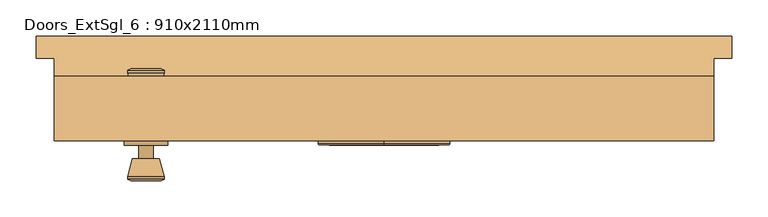
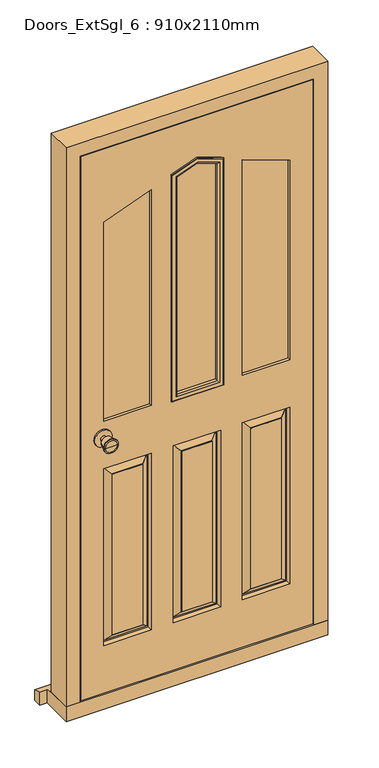
"""IFC4 building model written with IfcOpenShell, lengths in millimetres: door geometry, Doors_ExtSgl_6 : 910x2110mm."""

from ifc_helpers import new_model, si_unit, point, frame, frame_2d, origin, place, context, project, spatial, polyline, circle_curve, ellipse_curve, trimmed, segment, composite_curve, outline, extrude, faceted_brep, source, transform, mapped, element, save
from ifc_brep_helpers import plane_surface, cylinder_surface, revolved_surface, advanced_brep


def doors_extsgl_6_910x2110mm_5dc58899(model_context):
    return source(origin(), model_context, "Body", "SolidModel", [
        advanced_brep(
        [(-328.4666667, -18.4, 1000.0), (-318.4666667, -18.4, 1000.0), (-338.4666667, -18.4, 1000.0), (-307.9907991, -67.4, 1000.0), (-328.4666667, -67.4, 1000.0), (-348.9425342, -67.4, 1000.0), (-303.4666667, -65.5721319, 1000.0), (-353.4666667, -65.5721319, 1000.0), (-303.4666667, -62.1084537, 1000.0), (-353.4666667, -62.1084537, 1000.0), (-309.8304306, -37.4, 1000.0), (-347.1029027, -37.4, 1000.0), (-318.4666667, -37.4, 1000.0), (-338.4666667, -37.4, 1000.0)],
        [
            (0, 1),
            (1, 2, circle_curve(frame((-328.4666667, -18.4, 1000.0), z_axis=(0.0, 1.0, 0.0), x_axis=(-1.0, 0.0, 0.0)), 10.0)),
            (2, 0),
            (2, 1, circle_curve(frame((-328.4666667, -18.4, 1000.0), z_axis=(0.0, 1.0, 0.0), x_axis=(-1.0, 0.0, 0.0)), 10.0)),
            (3, 4),
            (4, 5),
            (5, 3, circle_curve(frame((-328.4666667, -67.4, 1000.0), z_axis=(0.0, -1.0, 0.0), x_axis=(-1.0, 0.0, 0.0)), 20.4758676)),
            (3, 5, circle_curve(frame((-328.4666667, -67.4, 1000.0), z_axis=(0.0, -1.0, 0.0), x_axis=(-1.0, 0.0, 0.0)), 20.4758676)),
            (6, 3),
            (5, 7),
            (7, 6, circle_curve(frame((-328.4666667, -65.5721319, 1000.0), z_axis=(0.0, -1.0, 0.0), x_axis=(-1.0, 0.0, 0.0)), 25.0)),
            (6, 7, circle_curve(frame((-328.4666667, -65.5721319, 1000.0), z_axis=(0.0, -1.0, 0.0), x_axis=(-1.0, 0.0, 0.0)), 25.0)),
            (8, 6),
            (7, 9),
            (9, 8, circle_curve(frame((-328.4666667, -62.1084537, 1000.0), z_axis=(0.0, -1.0, 0.0), x_axis=(-1.0, 0.0, 0.0)), 25.0)),
            (8, 9, circle_curve(frame((-328.4666667, -62.1084537, 1000.0), z_axis=(0.0, -1.0, 0.0), x_axis=(-1.0, 0.0, 0.0)), 25.0)),
            (10, 8),
            (9, 11),
            (11, 10, circle_curve(frame((-328.4666667, -37.4, 1000.0), z_axis=(0.0, -1.0, 0.0), x_axis=(-1.0, 0.0, 0.0)), 18.636236)),
            (10, 11, circle_curve(frame((-328.4666667, -37.4, 1000.0), z_axis=(0.0, -1.0, 0.0), x_axis=(-1.0, 0.0, 0.0)), 18.636236)),
            (12, 10),
            (11, 13),
            (13, 12, circle_curve(frame((-328.4666667, -37.4, 1000.0), z_axis=(0.0, -1.0, 0.0), x_axis=(-1.0, 0.0, 0.0)), 10.0)),
            (12, 13, circle_curve(frame((-328.4666667, -37.4, 1000.0), z_axis=(0.0, -1.0, 0.0), x_axis=(-1.0, 0.0, 0.0)), 10.0)),
            (1, 12),
            (13, 2),
        ],
        [
            plane_surface(frame((-328.4666667, -18.4, 1000.0), z_axis=(0.0, 1.0, 0.0), x_axis=(-1.0, 0.0, 0.0))),
            plane_surface(frame((-328.4666667, -67.4, 1000.0), z_axis=(0.0, -1.0, 0.0), x_axis=(-1.0, 0.0, 0.0))),
            revolved_surface(polyline([(-348.9425342, -67.4, 1000.0), (-353.4666667, -65.5721319, 1000.0)]), (-328.4666667, -18.4, 1000.0), (0.0, 1.0, 0.0)),
            cylinder_surface(frame((-328.4666667, -18.4, 1000.0), z_axis=(0.0, 1.0, 0.0), x_axis=(-1.0, 0.0, 0.0)), 25.0),
            revolved_surface(polyline([(-353.4666667, -62.1084537, 1000.0), (-347.1029027, -37.4, 1000.0)]), (-328.4666667, -18.4, 1000.0), (0.0, 1.0, 0.0)),
            plane_surface(frame((-328.4666667, -37.4, 1000.0), z_axis=(0.0, 1.0, 0.0), x_axis=(-1.0, 0.0, 0.0))),
            cylinder_surface(frame((-328.4666667, -18.4, 1000.0), z_axis=(0.0, 1.0, 0.0), x_axis=(-1.0, 0.0, 0.0)), 10.0),
        ],
        [
            (0, [[1, 2, 3]]),
            (0, [[-3, 4, -1]]),
            (1, [[5, 6, 7]]),
            (1, [[-6, -5, 8]]),
            (2, [[9, -7, 10, 11]]),
            (2, [[-10, -8, -9, 12]]),
            (3, [[13, -11, 14, 15]]),
            (3, [[-14, -12, -13, 16]]),
            (4, [[17, -15, 18, 19]]),
            (4, [[-18, -16, -17, 20]]),
            (5, [[21, -19, 22, 23]]),
            (5, [[-22, -20, -21, 24]]),
            (6, [[25, -23, 26, -2]]),
            (6, [[-26, -24, -25, -4]]),
        ],
    ),
        extrude(outline(composite_curve([segment(trimmed(circle_curve(frame_2d((1000.0, -328.4666667)), 30.0), [point((1000.0, -358.4666667))], [point((1000.0, -298.4666667))], False, "CARTESIAN"), True, "CONTINUOUS"), segment(trimmed(circle_curve(frame_2d((1000.0, -328.4666667)), 30.0), [point((1000.0, -298.4666667))], [point((1000.0, -358.4666667))], False, "CARTESIAN"), True, "CONTINUOUS")], self_intersect=False)), frame((0.0, -18.4, 0.0), z_axis=(0.0, 1.0, 0.0), x_axis=(0.0, 0.0, 1.0)), (0.0, 0.0, 1.0), 6.0),
        advanced_brep(
        [(-328.4666667, 37.6, 1000.0), (-338.4666667, 37.6, 1000.0), (-318.4666667, 37.6, 1000.0), (-307.9907991, 86.6, 1000.0), (-348.9425342, 86.6, 1000.0), (-328.4666667, 86.6, 1000.0), (-303.4666667, 84.7721319, 1000.0), (-353.4666667, 84.7721319, 1000.0), (-303.4666667, 81.3084537, 1000.0), (-353.4666667, 81.3084537, 1000.0), (-309.8304306, 56.6, 1000.0), (-347.1029027, 56.6, 1000.0), (-318.4666667, 56.6, 1000.0), (-338.4666667, 56.6, 1000.0)],
        [
            (0, 1),
            (1, 2, circle_curve(frame((-328.4666667, 37.6, 1000.0), z_axis=(0.0, -1.0, 0.0), x_axis=(-1.0, 0.0, 0.0)), 10.0)),
            (2, 0),
            (2, 1, circle_curve(frame((-328.4666667, 37.6, 1000.0), z_axis=(0.0, -1.0, 0.0), x_axis=(-1.0, 0.0, 0.0)), 10.0)),
            (3, 4, circle_curve(frame((-328.4666667, 86.6, 1000.0), z_axis=(0.0, 1.0, 0.0), x_axis=(-1.0, 0.0, 0.0)), 20.4758676)),
            (4, 5),
            (5, 3),
            (4, 3, circle_curve(frame((-328.4666667, 86.6, 1000.0), z_axis=(0.0, 1.0, 0.0), x_axis=(-1.0, 0.0, 0.0)), 20.4758676)),
            (6, 7, circle_curve(frame((-328.4666667, 84.7721319, 1000.0), z_axis=(0.0, 1.0, 0.0), x_axis=(-1.0, 0.0, 0.0)), 25.0)),
            (7, 4),
            (3, 6),
            (7, 6, circle_curve(frame((-328.4666667, 84.7721319, 1000.0), z_axis=(0.0, 1.0, 0.0), x_axis=(-1.0, 0.0, 0.0)), 25.0)),
            (8, 9, circle_curve(frame((-328.4666667, 81.3084537, 1000.0), z_axis=(0.0, 1.0, 0.0), x_axis=(-1.0, 0.0, 0.0)), 25.0)),
            (9, 7),
            (6, 8),
            (9, 8, circle_curve(frame((-328.4666667, 81.3084537, 1000.0), z_axis=(0.0, 1.0, 0.0), x_axis=(-1.0, 0.0, 0.0)), 25.0)),
            (10, 11, circle_curve(frame((-328.4666667, 56.6, 1000.0), z_axis=(0.0, 1.0, 0.0), x_axis=(-1.0, 0.0, 0.0)), 18.636236)),
            (11, 9),
            (8, 10),
            (11, 10, circle_curve(frame((-328.4666667, 56.6, 1000.0), z_axis=(0.0, 1.0, 0.0), x_axis=(-1.0, 0.0, 0.0)), 18.636236)),
            (12, 13, circle_curve(frame((-328.4666667, 56.6, 1000.0), z_axis=(0.0, 1.0, 0.0), x_axis=(-1.0, 0.0, 0.0)), 10.0)),
            (13, 11),
            (10, 12),
            (13, 12, circle_curve(frame((-328.4666667, 56.6, 1000.0), z_axis=(0.0, 1.0, 0.0), x_axis=(-1.0, 0.0, 0.0)), 10.0)),
            (1, 13),
            (12, 2),
        ],
        [
            plane_surface(frame((-328.4666667, 37.6, 1000.0), z_axis=(0.0, -1.0, 0.0), x_axis=(-1.0, 0.0, 0.0))),
            plane_surface(frame((-328.4666667, 86.6, 1000.0), z_axis=(0.0, 1.0, 0.0), x_axis=(-1.0, 0.0, 0.0))),
            revolved_surface(polyline([(-348.9425342, 86.6, 1000.0), (-353.4666667, 84.7721319, 1000.0)]), (-328.4666667, 37.6, 1000.0), (0.0, -1.0, 0.0)),
            cylinder_surface(frame((-328.4666667, 37.6, 1000.0), z_axis=(0.0, -1.0, 0.0), x_axis=(-1.0, 0.0, 0.0)), 25.0),
            revolved_surface(polyline([(-353.4666667, 81.3084537, 1000.0), (-347.1029027, 56.6, 1000.0)]), (-328.4666667, 37.6, 1000.0), (0.0, -1.0, 0.0)),
            plane_surface(frame((-328.4666667, 56.6, 1000.0), z_axis=(0.0, -1.0, 0.0), x_axis=(-1.0, 0.0, 0.0))),
            cylinder_surface(frame((-328.4666667, 37.6, 1000.0), z_axis=(0.0, -1.0, 0.0), x_axis=(-1.0, 0.0, 0.0)), 10.0),
        ],
        [
            (0, [[1, 2, 3]]),
            (0, [[-3, 4, -1]]),
            (1, [[5, 6, 7]]),
            (1, [[8, -7, -6]]),
            (2, [[9, 10, -5, 11]]),
            (2, [[12, -11, -8, -10]]),
            (3, [[13, 14, -9, 15]]),
            (3, [[16, -15, -12, -14]]),
            (4, [[17, 18, -13, 19]]),
            (4, [[20, -19, -16, -18]]),
            (5, [[21, 22, -17, 23]]),
            (5, [[24, -23, -20, -22]]),
            (6, [[-2, 25, -21, 26]]),
            (6, [[-4, -26, -24, -25]]),
        ],
    ),
        extrude(outline(composite_curve([segment(trimmed(circle_curve(frame_2d((1000.0, -328.4666667)), 30.0), [point((1000.0, -358.4666667))], [point((1000.0, -298.4666667))], False, "CARTESIAN"), True, "CONTINUOUS"), segment(trimmed(circle_curve(frame_2d((1000.0, -328.4666667)), 30.0), [point((1000.0, -298.4666667))], [point((1000.0, -358.4666667))], False, "CARTESIAN"), True, "CONTINUOUS")], self_intersect=False)), frame((0.0, 31.6, 0.0), z_axis=(0.0, 1.0, 0.0), x_axis=(0.0, 0.0, 1.0)), (0.0, 0.0, 1.0), 6.0),
        faceted_brep([(384.5333333, 76.6, 54.5), (455.0333333, 76.6, 54.5), (455.0333333, -12.4, 54.5), (406.5333333, -12.4, 54.5), (406.5333333, 34.6, 54.5), (384.5333333, 34.6, 54.5), (384.5333333, 76.6, 2039.5), (-384.4666667, 76.6, 2039.5), (-384.4666667, 76.6, 54.5), (-454.9666667, 76.6, 54.5), (-454.9666667, 76.6, 2110.0), (455.0333333, 76.6, 2110.0), (455.0333333, -12.4, 2110.0), (-454.9666667, -12.4, 2110.0), (-454.9666667, -12.4, 54.5), (-406.4666667, -12.4, 54.5), (-406.4666667, -12.4, 2061.5), (406.5333333, -12.4, 2061.5), (406.5333333, 34.6, 2061.5), (-406.4666667, 34.6, 2061.5), (-406.4666667, 34.6, 54.5), (-384.4666667, 34.6, 54.5), (-384.4666667, 34.6, 2039.5), (384.5333333, 34.6, 2039.5)], [[[0, 1, 2, 3, 4, 5]], [[1, 0, 6, 7, 8, 9, 10, 11]], [[2, 1, 11, 12]], [[3, 2, 12, 13, 14, 15, 16, 17]], [[4, 3, 17, 18]], [[5, 4, 18, 19, 20, 21, 22, 23]], [[0, 5, 23, 6]], [[8, 7, 22, 21]], [[9, 8, 21, 20, 15, 14]], [[10, 9, 14, 13]], [[16, 15, 20, 19]], [[11, 10, 13, 12]], [[17, 16, 19, 18]], [[7, 6, 23, 22]]]),
        faceted_brep([(403.5333333, -12.4, 58.5), (403.5333333, -12.4, 2058.5), (-404.3916961, -12.4, 2058.5), (-404.3916961, -12.4, 58.5), (-82.8, -12.4, 1058.5), (-82.8, -12.4, 1878.3511323), (0.0333333, -12.4, 1908.5), (82.8666667, -12.4, 1878.3511323), (82.8666667, -12.4, 1058.5), (323.5333333, -12.4, 1058.5), (157.8666667, -12.4, 1058.5), (157.8666667, -12.4, 1851.0533647), (323.5333333, -12.4, 1790.7556292), (-157.8, -12.4, 1851.0533647), (-157.8, -12.4, 1058.5), (-323.4666667, -12.4, 1058.5), (-323.4666667, -12.4, 1790.7556292), (-157.8, -12.4, 883.5), (-157.8, -12.4, 233.5), (-323.4666667, -12.4, 233.5), (-323.4666667, -12.4, 883.5), (323.5333333, -12.4, 883.5), (323.5333333, -12.4, 233.5), (157.8666667, -12.4, 233.5), (157.8666667, -12.4, 883.5), (82.8666667, -12.4, 883.5), (82.8666667, -12.4, 233.5), (-82.8, -12.4, 233.5), (-82.8, -12.4, 883.5), (-187.8, -12.4, 263.5), (-187.8, -12.4, 853.5), (-293.4666667, -12.4, 853.5), (-293.4666667, -12.4, 263.5), (293.5333333, -12.4, 263.5), (293.5333333, -12.4, 853.5), (187.8666667, -12.4, 853.5), (187.8666667, -12.4, 263.5), (52.8666667, -12.4, 263.5), (52.8666667, -12.4, 853.5), (-52.8, -12.4, 853.5), (-52.8, -12.4, 263.5), (403.5333333, 31.6, 58.5), (-404.3916961, 31.6, 58.5), (-404.3916961, 31.6, 2058.5), (403.5333333, 31.6, 2058.5), (-82.8, 31.6, 1058.5), (82.8666667, 31.6, 1058.5), (82.8666667, 31.6, 1878.3511323), (0.0333333, 31.6, 1908.5), (-82.8, 31.6, 1878.3511323), (323.5333333, 31.6, 1058.5), (323.5333333, 31.6, 1790.7556292), (157.8666667, 31.6, 1851.0533647), (157.8666667, 31.6, 1058.5), (-157.8, 31.6, 1851.0533647), (-323.4666667, 31.6, 1790.7556292), (-323.4666667, 31.6, 1058.5), (-157.8, 31.6, 1058.5), (157.8666667, 31.6, 883.5), (157.8666667, 31.6, 233.5), (323.5333333, 31.6, 233.5), (323.5333333, 31.6, 883.5), (-323.4666667, 31.6, 883.5), (-323.4666667, 31.6, 233.5), (-157.8, 31.6, 233.5), (-157.8, 31.6, 883.5), (-82.8, 31.6, 883.5), (-82.8, 31.6, 233.5), (82.8666667, 31.6, 233.5), (82.8666667, 31.6, 883.5), (187.8666667, 31.6, 263.5), (187.8666667, 31.6, 853.5), (293.5333333, 31.6, 853.5), (293.5333333, 31.6, 263.5), (-293.4666667, 31.6, 263.5), (-293.4666667, 31.6, 853.5), (-187.8, 31.6, 853.5), (-187.8, 31.6, 263.5), (-52.8, 31.6, 263.5), (-52.8, 31.6, 853.5), (52.8666667, 31.6, 853.5), (52.8666667, 31.6, 263.5), (160.8666667, 16.6, 880.5), (160.8666667, 16.6, 236.5), (185.8666667, 30.6, 855.5), (185.8666667, 30.6, 261.5), (165.8666667, 16.6, 241.5), (165.8666667, 16.6, 875.5), (187.8666667, 30.6, 263.5), (187.8666667, 30.6, 853.5), (320.5333333, 16.6, 236.5), (295.5333333, 30.6, 261.5), (315.5333333, 16.6, 241.5), (293.5333333, 30.6, 263.5), (320.5333333, 16.6, 880.5), (295.5333333, 30.6, 855.5), (315.5333333, 16.6, 875.5), (293.5333333, 30.6, 853.5), (-320.4666667, 16.6, 880.5), (-320.4666667, 16.6, 236.5), (-295.4666667, 30.6, 855.5), (-295.4666667, 30.6, 261.5), (-315.4666667, 16.6, 241.5), (-315.4666667, 16.6, 875.5), (-293.4666667, 30.6, 263.5), (-293.4666667, 30.6, 853.5), (-160.8, 16.6, 236.5), (-185.8, 30.6, 261.5), (-165.8, 16.6, 241.5), (-187.8, 30.6, 263.5), (-160.8, 16.6, 880.5), (-185.8, 30.6, 855.5), (-165.8, 16.6, 875.5), (-187.8, 30.6, 853.5), (-187.8, -11.4, 263.5), (-187.8, -11.4, 853.5), (-165.8, 2.6, 241.5), (-165.8, 2.6, 875.5), (-185.8, -11.4, 855.5), (-185.8, -11.4, 261.5), (-160.8, 2.6, 880.5), (-160.8, 2.6, 236.5), (-293.4666667, -11.4, 853.5), (-315.4666667, 2.6, 875.5), (-295.4666667, -11.4, 855.5), (-320.4666667, 2.6, 880.5), (-293.4666667, -11.4, 263.5), (-315.4666667, 2.6, 241.5), (-295.4666667, -11.4, 261.5), (-320.4666667, 2.6, 236.5), (320.5333333, 2.6, 880.5), (320.5333333, 2.6, 236.5), (295.5333333, -11.4, 855.5), (295.5333333, -11.4, 261.5), (315.5333333, 2.6, 241.5), (315.5333333, 2.6, 875.5), (293.5333333, -11.4, 263.5), (293.5333333, -11.4, 853.5), (160.8666667, 2.6, 236.5), (185.8666667, -11.4, 261.5), (165.8666667, 2.6, 241.5), (187.8666667, -11.4, 263.5), (160.8666667, 2.6, 880.5), (185.8666667, -11.4, 855.5), (165.8666667, 2.6, 875.5), (187.8666667, -11.4, 853.5), (-52.8, 30.6, 263.5), (-52.8, 30.6, 853.5), (-74.8, 16.6, 241.5), (-74.8, 16.6, 875.5), (-54.8, 30.6, 855.5), (-54.8, 30.6, 261.5), (-79.8, 16.6, 880.5), (-79.8, 16.6, 236.5), (52.8666667, 30.6, 853.5), (74.8666667, 16.6, 875.5), (54.8666667, 30.6, 855.5), (79.8666667, 16.6, 880.5), (52.8666667, 30.6, 263.5), (74.8666667, 16.6, 241.5), (54.8666667, 30.6, 261.5), (79.8666667, 16.6, 236.5), (79.8666667, 2.6, 880.5), (79.8666667, 2.6, 236.5), (54.8666667, -11.4, 855.5), (54.8666667, -11.4, 261.5), (74.8666667, 2.6, 241.5), (74.8666667, 2.6, 875.5), (52.8666667, -11.4, 263.5), (52.8666667, -11.4, 853.5), (-79.8, 2.6, 236.5), (-54.8, -11.4, 261.5), (-74.8, 2.6, 241.5), (-52.8, -11.4, 263.5), (-79.8, 2.6, 880.5), (-54.8, -11.4, 855.5), (-74.8, 2.6, 875.5), (-52.8, -11.4, 853.5)], [[[0, 1, 2, 3], [4, 5, 6, 7, 8], [9, 10, 11, 12], [13, 14, 15, 16], [17, 18, 19, 20], [21, 22, 23, 24], [25, 26, 27, 28]], [[29, 30, 31, 32]], [[33, 34, 35, 36]], [[37, 38, 39, 40]], [[41, 42, 43, 44], [45, 46, 47, 48, 49], [50, 51, 52, 53], [54, 55, 56, 57], [58, 59, 60, 61], [62, 63, 64, 65], [66, 67, 68, 69]], [[70, 71, 72, 73]], [[74, 75, 76, 77]], [[78, 79, 80, 81]], [[1, 0, 41, 44]], [[2, 1, 44, 43]], [[3, 2, 43, 42]], [[0, 3, 42, 41]], [[5, 4, 45, 49]], [[6, 5, 49, 48]], [[7, 6, 48, 47]], [[8, 7, 47, 46]], [[4, 8, 46, 45]], [[10, 9, 50, 53]], [[11, 10, 53, 52]], [[12, 11, 52, 51]], [[9, 12, 51, 50]], [[14, 13, 54, 57]], [[15, 14, 57, 56]], [[16, 15, 56, 55]], [[13, 16, 55, 54]], [[82, 83, 59, 58]], [[84, 85, 86, 87]], [[70, 88, 89, 71]], [[59, 83, 90, 60]], [[86, 85, 91, 92]], [[88, 70, 73, 93]], [[60, 90, 94, 61]], [[92, 91, 95, 96]], [[93, 73, 72, 97]], [[82, 58, 61, 94]], [[83, 82, 94, 90], [87, 86, 92, 96]], [[84, 87, 96, 95]], [[85, 84, 95, 91], [89, 88, 93, 97]], [[71, 89, 97, 72]], [[98, 99, 63, 62]], [[100, 101, 102, 103]], [[74, 104, 105, 75]], [[63, 99, 106, 64]], [[102, 101, 107, 108]], [[104, 74, 77, 109]], [[64, 106, 110, 65]], [[108, 107, 111, 112]], [[109, 77, 76, 113]], [[98, 62, 65, 110]], [[99, 98, 110, 106], [103, 102, 108, 112]], [[100, 103, 112, 111]], [[101, 100, 111, 107], [105, 104, 109, 113]], [[75, 105, 113, 76]], [[114, 115, 30, 29]], [[116, 117, 118, 119]], [[17, 120, 121, 18]], [[30, 115, 122, 31]], [[118, 117, 123, 124]], [[120, 17, 20, 125]], [[31, 122, 126, 32]], [[124, 123, 127, 128]], [[125, 20, 19, 129]], [[114, 29, 32, 126]], [[119, 118, 124, 128], [115, 114, 126, 122]], [[116, 119, 128, 127]], [[121, 120, 125, 129], [117, 116, 127, 123]], [[18, 121, 129, 19]], [[130, 131, 22, 21]], [[132, 133, 134, 135]], [[33, 136, 137, 34]], [[22, 131, 138, 23]], [[134, 133, 139, 140]], [[136, 33, 36, 141]], [[23, 138, 142, 24]], [[140, 139, 143, 144]], [[141, 36, 35, 145]], [[130, 21, 24, 142]], [[131, 130, 142, 138], [135, 134, 140, 144]], [[132, 135, 144, 143]], [[133, 132, 143, 139], [137, 136, 141, 145]], [[34, 137, 145, 35]], [[146, 147, 79, 78]], [[148, 149, 150, 151]], [[66, 152, 153, 67]], [[79, 147, 154, 80]], [[150, 149, 155, 156]], [[152, 66, 69, 157]], [[80, 154, 158, 81]], [[156, 155, 159, 160]], [[157, 69, 68, 161]], [[146, 78, 81, 158]], [[151, 150, 156, 160], [147, 146, 158, 154]], [[148, 151, 160, 159]], [[153, 152, 157, 161], [149, 148, 159, 155]], [[67, 153, 161, 68]], [[162, 163, 26, 25]], [[164, 165, 166, 167]], [[37, 168, 169, 38]], [[26, 163, 170, 27]], [[166, 165, 171, 172]], [[168, 37, 40, 173]], [[27, 170, 174, 28]], [[172, 171, 175, 176]], [[173, 40, 39, 177]], [[162, 25, 28, 174]], [[163, 162, 174, 170], [167, 166, 172, 176]], [[164, 167, 176, 175]], [[165, 164, 175, 171], [169, 168, 173, 177]], [[38, 169, 177, 39]]]),
        faceted_brep([(480.0333333, 131.6, 0.0), (480.0333333, 131.6, 38.5947221), (480.0333333, 101.6, 47.2703282), (480.0333333, 101.6, 0.0), (-479.9666667, 131.6, 38.5947221), (-479.9666667, 131.6, 0.0), (-479.9666667, 101.6, 0.0), (-479.9666667, 101.6, 47.2703282), (455.0333333, 101.6, 0.0), (455.0333333, -12.4, 0.0), (-454.9666667, -12.4, 0.0), (-454.9666667, 101.6, 0.0), (-454.9666667, 101.6, 47.2703282), (-454.9666667, 76.6, 54.5), (455.0333333, 76.6, 54.5), (455.0333333, 101.6, 47.2703282), (-454.9666667, -12.4, 54.5), (455.0333333, -12.4, 54.5)], [[[0, 1, 2, 3]], [[4, 5, 6, 7]], [[5, 0, 3, 8, 9, 10, 11, 6]], [[1, 0, 5, 4]], [[1, 4, 7, 12, 13, 14, 15, 2]], [[13, 16, 17, 14]], [[16, 10, 9, 17]], [[12, 11, 10, 16, 13]], [[11, 12, 7, 6]], [[8, 15, 14, 17, 9]], [[15, 8, 3, 2]]]),
        extrude(outline(polyline([(1058.5, -82.8), (1058.5, 82.8666667), (1878.3511323, 82.8666667), (1908.5, 0.0333333), (1878.3511323, -82.8), (1058.5, -82.8)])), frame((0.0, -2.4, 0.0), z_axis=(0.0, 1.0, 0.0), x_axis=(0.0, 0.0, 1.0)), (0.0, 0.0, 1.0), 24.0),
        extrude(outline(polyline([(1790.7556292, 323.5333333), (1851.0533647, 157.8666667), (1058.5, 157.8666667), (1058.5, 323.5333333), (1790.7556292, 323.5333333)])), frame((0.0, -2.4, 0.0), z_axis=(0.0, 1.0, 0.0), x_axis=(0.0, 0.0, 1.0)), (0.0, 0.0, 1.0), 24.0),
        extrude(outline(polyline([(1058.5, -157.8), (1851.0533647, -157.8), (1790.7556292, -323.4666667), (1058.5, -323.4666667), (1058.5, -157.8)])), frame((0.0, -2.4, 0.0), z_axis=(0.0, 1.0, 0.0), x_axis=(0.0, 0.0, 1.0)), (0.0, 0.0, 1.0), 24.0),
        advanced_brep(
        [(-90.8, 35.6, 1050.5), (-90.8, 31.6, 1050.5), (-90.8, 31.6, 1883.9527926), (-90.8, 35.6, 1883.9527926), (-88.8, 37.6, 1052.5), (-88.8, 37.6, 1882.5523775), (-70.8, 32.6, 1070.5), (-75.8, 37.6, 1065.5), (-75.8, 37.6, 1873.4496795), (-70.8, 32.6, 1869.9486418), (-70.8, 21.6, 1070.5), (-70.8, 21.6, 1869.9486418), (-82.8, 31.6, 1058.5), (-82.8, 21.6, 1058.5), (-82.8, 21.6, 1878.3511323), (-82.8, 31.6, 1878.3511323), (0.0333333, 31.6, 1917.0134222), (0.0333333, 35.6, 1917.0134222), (0.0333333, 37.6, 1914.8850666), (0.0333333, 37.6, 1901.0507556), (0.0333333, 32.6, 1895.7298667), (0.0333333, 21.6, 1895.7298667), (0.0333333, 21.6, 1908.5), (0.0333333, 31.6, 1908.5), (90.8666667, 31.6, 1883.9527926), (90.8666667, 35.6, 1883.9527926), (88.8666667, 37.6, 1882.5523775), (88.8666667, 37.6, 1052.5), (75.8666667, 37.6, 1873.4496795), (75.8666667, 37.6, 1065.5), (70.8666667, 32.6, 1869.9486418), (70.8666667, 21.6, 1869.9486418), (82.8666667, 21.6, 1878.3511323), (82.8666667, 21.6, 1058.5), (70.8666667, 21.6, 1070.5), (82.8666667, 31.6, 1878.3511323), (90.8666667, 31.6, 1050.5), (82.8666667, 31.6, 1058.5), (90.8666667, 35.6, 1050.5), (70.8666667, 32.6, 1070.5)],
        [
            (0, 1),
            (1, 2),
            (2, 3),
            (3, 0),
            (4, 0, ellipse_curve(frame((-88.8, 35.6, 1052.5), z_axis=(-0.7071067811865476, 0.0, 0.7071067811865474), x_axis=(-0.7071067811865472, 0.0, -0.7071067811865478)), 2.8284271, 2.0)),
            (3, 5, ellipse_curve(frame((-88.8, 35.6, 1882.5523775), z_axis=(-0.5735764363510456, 0.0, -0.8191520442889918), x_axis=(0.8191520442889916, 0.0, -0.5735764363510464)), 2.4415492, 2.0)),
            (5, 4),
            (6, 7, ellipse_curve(frame((-75.8, 32.6, 1065.5), z_axis=(-0.7071067811865476, 0.0, 0.7071067811865474), x_axis=(-0.7071067811865472, 0.0, -0.7071067811865478)), 7.0710678, 5.0)),
            (7, 8),
            (8, 9, ellipse_curve(frame((-75.8, 32.6, 1873.4496795), z_axis=(-0.5735764363510456, 0.0, -0.8191520442889918), x_axis=(0.8191520442889916, 0.0, -0.5735764363510464)), 6.1038729, 5.0)),
            (9, 6),
            (10, 6),
            (9, 11),
            (11, 10),
            (12, 13),
            (13, 14),
            (14, 15),
            (15, 12),
            (2, 16),
            (16, 17),
            (17, 3),
            (17, 18, ellipse_curve(frame((0.0333333, 35.6, 1914.8850666), z_axis=(-1.0, 0.0, 0.0), x_axis=(0.0, 0.0, -1.0)), 2.1283555, 2.0)),
            (18, 5),
            (8, 19),
            (19, 20, ellipse_curve(frame((0.0333333, 32.6, 1901.0507556), z_axis=(-1.0, 0.0, 0.0), x_axis=(0.0, 0.0, -1.0)), 5.3208889, 5.0)),
            (20, 9),
            (20, 21),
            (21, 11),
            (14, 22),
            (22, 23),
            (23, 15),
            (16, 24),
            (24, 25),
            (25, 17),
            (25, 26, ellipse_curve(frame((88.8666667, 35.6, 1882.5523775), z_axis=(-0.573576436351046, 0.0, 0.8191520442889917), x_axis=(-0.8191520442889921, 0.0, -0.5735764363510458)), 2.4415492, 2.0)),
            (26, 18),
            (26, 27),
            (27, 4),
            (28, 19),
            (7, 29),
            (29, 28),
            (28, 30, ellipse_curve(frame((75.8666667, 32.6, 1873.4496795), z_axis=(-0.573576436351046, 0.0, 0.8191520442889917), x_axis=(-0.8191520442889921, 0.0, -0.5735764363510458)), 6.1038729, 5.0)),
            (30, 20),
            (30, 31),
            (31, 21),
            (32, 22),
            (13, 33),
            (33, 32),
            (31, 34),
            (34, 10),
            (32, 35),
            (35, 23),
            (1, 36),
            (36, 24),
            (35, 37),
            (37, 12),
            (36, 38),
            (38, 25),
            (38, 27, ellipse_curve(frame((88.8666667, 35.6, 1052.5), z_axis=(0.7071067811865475, 0.0, 0.7071067811865476), x_axis=(-0.7071067811865475, 0.0, 0.7071067811865475)), 2.8284271, 2.0)),
            (29, 39, ellipse_curve(frame((75.8666667, 32.6, 1065.5), z_axis=(0.7071067811865475, 0.0, 0.7071067811865476), x_axis=(-0.7071067811865475, 0.0, 0.7071067811865475)), 7.0710678, 5.0)),
            (39, 30),
            (39, 34),
            (33, 37),
            (0, 38),
            (6, 39),
        ],
        [
            plane_surface(frame((-90.8, 31.6, 1050.5), z_axis=(-1.0, 0.0, 0.0), x_axis=(0.0, 0.0, 1.0))),
            cylinder_surface(frame((-88.8, 35.6, 1058.5), z_axis=(0.0, 0.0, -1.0), x_axis=(-1.0, 0.0, 0.0)), 2.0),
            cylinder_surface(frame((-75.8, 32.6, 1058.5), z_axis=(0.0, 0.0, -1.0), x_axis=(-1.0, 0.0, 0.0)), 5.0),
            plane_surface(frame((-70.8, 32.6, 1070.5), z_axis=(1.0, 0.0, 0.0), x_axis=(0.0, 0.0, 1.0))),
            plane_surface(frame((-82.8, 21.6, 1058.5), z_axis=(-1.0, 0.0, 0.0), x_axis=(0.0, 0.0, 1.0))),
            plane_surface(frame((-90.8, 31.6, 1883.9527926), z_axis=(-0.34202014332566827, 0.0, 0.9396926207859086), x_axis=(0.9396926207859086, 0.0, 0.34202014332566827))),
            cylinder_surface(frame((-84.8521209, 35.6, 1883.989288), z_axis=(-0.9396926207859082, 0.0, -0.34202014332566943), x_axis=(-0.34202014332566943, 0.0, 0.9396926207859082)), 2.0),
            cylinder_surface(frame((-80.405859, 32.6, 1871.7732839), z_axis=(-0.9396926207859082, 0.0, -0.34202014332566943), x_axis=(-0.34202014332566943, 0.0, 0.9396926207859082)), 5.0),
            plane_surface(frame((-70.8, 32.6, 1869.9486418), z_axis=(0.34202014332567066, 0.0, -0.9396926207859078), x_axis=(0.9396926207859078, 0.0, 0.34202014332567066))),
            plane_surface(frame((-82.8, 21.6, 1878.3511323), z_axis=(-0.3420201433256691, 0.0, 0.9396926207859083), x_axis=(0.9396926207859083, 0.0, 0.3420201433256691))),
            plane_surface(frame((0.0333333, 31.6, 1917.0134222), z_axis=(0.342020143325669, 0.0, 0.9396926207859083), x_axis=(0.9396926207859083, 0.0, -0.342020143325669))),
            cylinder_surface(frame((2.0854542, 35.6, 1914.1381557), z_axis=(-0.9396926207859084, 0.0, 0.342020143325669), x_axis=(0.342020143325669, 0.0, 0.9396926207859084)), 2.0),
            plane_surface(frame((0.0333333, 37.6, 1914.8850666), z_axis=(0.0, 1.0000000000000002, 0.0), x_axis=(0.9396926207859082, 0.0, -0.34202014332566943))),
            cylinder_surface(frame((-2.3608077, 32.6, 1901.9221517), z_axis=(-0.9396926207859084, 0.0, 0.342020143325669), x_axis=(0.342020143325669, 0.0, 0.9396926207859084)), 5.0),
            plane_surface(frame((0.0333333, 32.6, 1895.7298667), z_axis=(-0.34202014332566794, 0.0, -0.9396926207859086), x_axis=(0.9396926207859086, 0.0, -0.34202014332566794))),
            plane_surface(frame((0.0333333, 21.6, 1895.7298667), z_axis=(0.0, -1.0000000000000002, 0.0), x_axis=(0.9396926207859088, 0.0, -0.3420201433256679))),
            plane_surface(frame((0.0333333, 21.6, 1908.5), z_axis=(0.342020143325668, 0.0, 0.9396926207859086), x_axis=(0.9396926207859086, 0.0, -0.342020143325668))),
            plane_surface(frame((0.0333333, 31.6, 1908.5), z_axis=(0.0, -1.0, 0.0), x_axis=(0.9396926207859086, 0.0, -0.342020143325668))),
            plane_surface(frame((90.8666667, 31.6, 1883.9527926), z_axis=(1.0, 0.0, 0.0), x_axis=(0.0, 0.0, -1.0))),
            cylinder_surface(frame((88.8666667, 35.6, 1878.3511323), z_axis=(0.0, 0.0, 1.0), x_axis=(1.0, 0.0, 0.0)), 2.0),
            cylinder_surface(frame((75.8666667, 32.6, 1878.3511323), z_axis=(0.0, 0.0, 1.0), x_axis=(1.0, 0.0, 0.0)), 5.0),
            plane_surface(frame((70.8666667, 32.6, 1869.9486418), z_axis=(-1.0, 0.0, 0.0), x_axis=(0.0, 0.0, -1.0))),
            plane_surface(frame((82.8666667, 21.6, 1878.3511323), z_axis=(1.0, 0.0, 0.0), x_axis=(0.0, 0.0, -1.0))),
            plane_surface(frame((90.8666667, 31.6, 1050.5), z_axis=(0.0, 0.0, -1.0), x_axis=(-1.0, 0.0, 0.0))),
            cylinder_surface(frame((82.8666667, 35.6, 1052.5), z_axis=(1.0, 0.0, 0.0), x_axis=(0.0, 0.0, -1.0)), 2.0),
            cylinder_surface(frame((82.8666667, 32.6, 1065.5), z_axis=(1.0, 0.0, 0.0), x_axis=(0.0, 0.0, -1.0)), 5.0),
            plane_surface(frame((70.8666667, 32.6, 1070.5), z_axis=(0.0, 0.0, 1.0), x_axis=(-1.0, 0.0, 0.0))),
            plane_surface(frame((82.8666667, 21.6, 1058.5), z_axis=(0.0, 0.0, -1.0), x_axis=(-1.0, 0.0, 0.0))),
        ],
        [
            (0, [[1, 2, 3, 4]]),
            (1, [[5, -4, 6, 7]]),
            (2, [[8, 9, 10, 11]]),
            (3, [[12, -11, 13, 14]]),
            (4, [[15, 16, 17, 18]]),
            (5, [[-3, 19, 20, 21]]),
            (6, [[-6, -21, 22, 23]]),
            (7, [[-10, 24, 25, 26]]),
            (8, [[-13, -26, 27, 28]]),
            (9, [[-17, 29, 30, 31]]),
            (10, [[-20, 32, 33, 34]]),
            (11, [[-22, -34, 35, 36]]),
            (12, [[-7, -23, -36, 37, 38], [39, -24, -9, 40, 41]]),
            (13, [[-25, -39, 42, 43]]),
            (14, [[-27, -43, 44, 45]]),
            (15, [[46, -29, -16, 47, 48], [-14, -28, -45, 49, 50]]),
            (16, [[-30, -46, 51, 52]]),
            (17, [[-32, -19, -2, 53, 54], [-18, -31, -52, 55, 56]]),
            (18, [[-33, -54, 57, 58]]),
            (19, [[-35, -58, 59, -37]]),
            (20, [[-42, -41, 60, 61]]),
            (21, [[-44, -61, 62, -49]]),
            (22, [[-51, -48, 63, -55]]),
            (23, [[-57, -53, -1, 64]]),
            (24, [[-59, -64, -5, -38]]),
            (25, [[-60, -40, -8, 65]]),
            (26, [[-62, -65, -12, -50]]),
            (27, [[-63, -47, -15, -56]]),
        ],
    ),
        advanced_brep(
        [(90.8666667, -16.4, 1050.5), (90.8666667, -12.4, 1050.5), (90.8666667, -12.4, 1883.9527926), (90.8666667, -16.4, 1883.9527926), (88.8666667, -18.4, 1052.5), (88.8666667, -18.4, 1882.5523775), (70.8666667, -13.4, 1070.5), (75.8666667, -18.4, 1065.5), (75.8666667, -18.4, 1873.4496795), (70.8666667, -13.4, 1869.9486418), (70.8666667, -2.4, 1070.5), (70.8666667, -2.4, 1869.9486418), (82.8666667, -12.4, 1058.5), (82.8666667, -2.4, 1058.5), (82.8666667, -2.4, 1878.3511323), (82.8666667, -12.4, 1878.3511323), (0.0333333, -12.4, 1917.0134222), (0.0333333, -16.4, 1917.0134222), (0.0333333, -18.4, 1914.8850666), (0.0333333, -18.4, 1901.0507556), (0.0333333, -13.4, 1895.7298667), (0.0333333, -2.4, 1895.7298667), (0.0333333, -2.4, 1908.5), (0.0333333, -12.4, 1908.5), (-90.8, -12.4, 1883.9527926), (-90.8, -16.4, 1883.9527926), (-88.8, -18.4, 1882.5523775), (-88.8, -18.4, 1052.5), (-75.8, -18.4, 1873.4496795), (-75.8, -18.4, 1065.5), (-70.8, -13.4, 1869.9486418), (-70.8, -2.4, 1869.9486418), (-82.8, -2.4, 1878.3511323), (-82.8, -2.4, 1058.5), (-70.8, -2.4, 1070.5), (-82.8, -12.4, 1878.3511323), (-90.8, -12.4, 1050.5), (-82.8, -12.4, 1058.5), (-90.8, -16.4, 1050.5), (-70.8, -13.4, 1070.5)],
        [
            (0, 1),
            (1, 2),
            (2, 3),
            (3, 0),
            (4, 0, ellipse_curve(frame((88.8666667, -16.4, 1052.5), z_axis=(0.7071067811865472, 0.0, 0.7071067811865478), x_axis=(0.7071067811865478, 0.0, -0.7071067811865474)), 2.8284271, 2.0)),
            (3, 5, ellipse_curve(frame((88.8666667, -16.4, 1882.5523775), z_axis=(0.5735764363510463, 0.0, -0.8191520442889916), x_axis=(-0.8191520442889915, 0.0, -0.5735764363510464)), 2.4415492, 2.0)),
            (5, 4),
            (6, 7, ellipse_curve(frame((75.8666667, -13.4, 1065.5), z_axis=(0.7071067811865472, 0.0, 0.7071067811865478), x_axis=(0.7071067811865478, 0.0, -0.7071067811865474)), 7.0710678, 5.0)),
            (7, 8),
            (8, 9, ellipse_curve(frame((75.8666667, -13.4, 1873.4496795), z_axis=(0.5735764363510463, 0.0, -0.8191520442889916), x_axis=(-0.8191520442889915, 0.0, -0.5735764363510464)), 6.1038729, 5.0)),
            (9, 6),
            (10, 6),
            (9, 11),
            (11, 10),
            (12, 13),
            (13, 14),
            (14, 15),
            (15, 12),
            (2, 16),
            (16, 17),
            (17, 3),
            (17, 18, ellipse_curve(frame((0.0333333, -16.4, 1914.8850666), z_axis=(1.0, 0.0, 0.0), x_axis=(0.0, 0.0, -1.0)), 2.1283555, 2.0)),
            (18, 5),
            (8, 19),
            (19, 20, ellipse_curve(frame((0.0333333, -13.4, 1901.0507556), z_axis=(1.0, 0.0, 0.0), x_axis=(0.0, 0.0, -1.0)), 5.3208889, 5.0)),
            (20, 9),
            (20, 21),
            (21, 11),
            (14, 22),
            (22, 23),
            (23, 15),
            (16, 24),
            (24, 25),
            (25, 17),
            (25, 26, ellipse_curve(frame((-88.8, -16.4, 1882.5523775), z_axis=(0.5735764363510456, 0.0, 0.8191520442889921), x_axis=(0.819152044288992, 0.0, -0.5735764363510455)), 2.4415492, 2.0)),
            (26, 18),
            (26, 27),
            (27, 4),
            (28, 19),
            (7, 29),
            (29, 28),
            (28, 30, ellipse_curve(frame((-75.8, -13.4, 1873.4496795), z_axis=(0.5735764363510456, 0.0, 0.8191520442889921), x_axis=(0.819152044288992, 0.0, -0.5735764363510455)), 6.1038729, 5.0)),
            (30, 20),
            (30, 31),
            (31, 21),
            (32, 22),
            (13, 33),
            (33, 32),
            (31, 34),
            (34, 10),
            (32, 35),
            (35, 23),
            (1, 36),
            (36, 24),
            (35, 37),
            (37, 12),
            (36, 38),
            (38, 25),
            (38, 27, ellipse_curve(frame((-88.8, -16.4, 1052.5), z_axis=(-0.7071067811865479, 0.0, 0.707106781186547), x_axis=(0.7071067811865468, 0.0, 0.7071067811865481)), 2.8284271, 2.0)),
            (29, 39, ellipse_curve(frame((-75.8, -13.4, 1065.5), z_axis=(-0.7071067811865479, 0.0, 0.707106781186547), x_axis=(0.7071067811865468, 0.0, 0.7071067811865481)), 7.0710678, 5.0)),
            (39, 30),
            (39, 34),
            (33, 37),
            (0, 38),
            (6, 39),
        ],
        [
            plane_surface(frame((90.8666667, -12.4, 1050.5), z_axis=(1.0, 0.0, 0.0), x_axis=(0.0, 0.0, 1.0))),
            cylinder_surface(frame((88.8666667, -16.4, 1058.5), z_axis=(0.0, 0.0, -1.0), x_axis=(1.0, 0.0, 0.0)), 2.0),
            cylinder_surface(frame((75.8666667, -13.4, 1058.5), z_axis=(0.0, 0.0, -1.0), x_axis=(1.0, 0.0, 0.0)), 5.0),
            plane_surface(frame((70.8666667, -13.4, 1070.5), z_axis=(-1.0, 0.0, 0.0), x_axis=(0.0, 0.0, 1.0))),
            plane_surface(frame((82.8666667, -2.4, 1058.5), z_axis=(1.0, 0.0, 0.0), x_axis=(0.0, 0.0, 1.0))),
            plane_surface(frame((90.8666667, -12.4, 1883.9527926), z_axis=(0.3420201433256677, 0.0, 0.9396926207859089), x_axis=(-0.9396926207859089, 0.0, 0.3420201433256677))),
            cylinder_surface(frame((84.9187875, -16.4, 1883.989288), z_axis=(0.9396926207859085, 0.0, -0.34202014332566855), x_axis=(0.34202014332566855, 0.0, 0.9396926207859085)), 2.0),
            cylinder_surface(frame((80.4725257, -13.4, 1871.7732839), z_axis=(0.9396926207859085, 0.0, -0.34202014332566855), x_axis=(0.34202014332566855, 0.0, 0.9396926207859085)), 5.0),
            plane_surface(frame((70.8666667, -13.4, 1869.9486418), z_axis=(-0.3420201433256698, 0.0, -0.939692620785908), x_axis=(-0.939692620785908, 0.0, 0.3420201433256698))),
            plane_surface(frame((82.8666667, -2.4, 1878.3511323), z_axis=(0.34202014332566855, 0.0, 0.9396926207859085), x_axis=(-0.9396926207859085, 0.0, 0.34202014332566855))),
            plane_surface(frame((0.0333333, -12.4, 1917.0134222), z_axis=(-0.3420201433256698, 0.0, 0.9396926207859081), x_axis=(-0.9396926207859081, 0.0, -0.3420201433256698))),
            cylinder_surface(frame((-2.0187875, -16.4, 1914.1381557), z_axis=(0.9396926207859082, 0.0, 0.3420201433256693), x_axis=(-0.3420201433256693, 0.0, 0.9396926207859082)), 2.0),
            plane_surface(frame((0.0333333, -18.4, 1914.8850666), z_axis=(0.0, -1.0, 0.0), x_axis=(-0.939692620785908, 0.0, -0.34202014332566993))),
            cylinder_surface(frame((2.4274743, -13.4, 1901.9221517), z_axis=(0.9396926207859082, 0.0, 0.3420201433256693), x_axis=(-0.3420201433256693, 0.0, 0.9396926207859082)), 5.0),
            plane_surface(frame((0.0333333, -13.4, 1895.7298667), z_axis=(0.34202014332566916, 0.0, -0.9396926207859082), x_axis=(-0.9396926207859082, 0.0, -0.34202014332566916))),
            plane_surface(frame((0.0333333, -2.4, 1895.7298667), z_axis=(0.0, 1.0, 0.0), x_axis=(-0.9396926207859082, 0.0, -0.3420201433256692))),
            plane_surface(frame((0.0333333, -2.4, 1908.5), z_axis=(-0.3420201433256711, 0.0, 0.9396926207859075), x_axis=(-0.9396926207859075, 0.0, -0.3420201433256711))),
            plane_surface(frame((0.0333333, -12.4, 1908.5), z_axis=(0.0, 1.0, 0.0), x_axis=(-0.9396926207859075, 0.0, -0.3420201433256711))),
            plane_surface(frame((-90.8, -12.4, 1883.9527926), z_axis=(-1.0, 0.0, 0.0), x_axis=(0.0, 0.0, -1.0))),
            cylinder_surface(frame((-88.8, -16.4, 1878.3511323), z_axis=(0.0, 0.0, 1.0), x_axis=(-1.0, 0.0, 0.0)), 2.0),
            cylinder_surface(frame((-75.8, -13.4, 1878.3511323), z_axis=(0.0, 0.0, 1.0), x_axis=(-1.0, 0.0, 0.0)), 5.0),
            plane_surface(frame((-70.8, -13.4, 1869.9486418), z_axis=(1.0, 0.0, 0.0), x_axis=(0.0, 0.0, -1.0))),
            plane_surface(frame((-82.8, -2.4, 1878.3511323), z_axis=(-1.0, 0.0, 0.0), x_axis=(0.0, 0.0, -1.0))),
            plane_surface(frame((-90.8, -12.4, 1050.5), z_axis=(0.0, 0.0, -1.0), x_axis=(1.0, 0.0, 0.0))),
            cylinder_surface(frame((-82.8, -16.4, 1052.5), z_axis=(-1.0, 0.0, 0.0), x_axis=(0.0, 0.0, -1.0)), 2.0),
            cylinder_surface(frame((-82.8, -13.4, 1065.5), z_axis=(-1.0, 0.0, 0.0), x_axis=(0.0, 0.0, -1.0)), 5.0),
            plane_surface(frame((-70.8, -13.4, 1070.5), z_axis=(0.0, 0.0, 1.0), x_axis=(1.0, 0.0, 0.0))),
            plane_surface(frame((-82.8, -2.4, 1058.5), z_axis=(0.0, 0.0, -1.0), x_axis=(1.0, 0.0, 0.0))),
        ],
        [
            (0, [[1, 2, 3, 4]]),
            (1, [[5, -4, 6, 7]]),
            (2, [[8, 9, 10, 11]]),
            (3, [[12, -11, 13, 14]]),
            (4, [[15, 16, 17, 18]]),
            (5, [[-3, 19, 20, 21]]),
            (6, [[-6, -21, 22, 23]]),
            (7, [[-10, 24, 25, 26]]),
            (8, [[-13, -26, 27, 28]]),
            (9, [[-17, 29, 30, 31]]),
            (10, [[-20, 32, 33, 34]]),
            (11, [[-22, -34, 35, 36]]),
            (12, [[-7, -23, -36, 37, 38], [39, -24, -9, 40, 41]]),
            (13, [[-25, -39, 42, 43]]),
            (14, [[-27, -43, 44, 45]]),
            (15, [[46, -29, -16, 47, 48], [-14, -28, -45, 49, 50]]),
            (16, [[-30, -46, 51, 52]]),
            (17, [[-32, -19, -2, 53, 54], [-18, -31, -52, 55, 56]]),
            (18, [[-33, -54, 57, 58]]),
            (19, [[-35, -58, 59, -37]]),
            (20, [[-42, -41, 60, 61]]),
            (21, [[-44, -61, 62, -49]]),
            (22, [[-51, -48, 63, -55]]),
            (23, [[-57, -53, -1, 64]]),
            (24, [[-59, -64, -5, -38]]),
            (25, [[-60, -40, -8, 65]]),
            (26, [[-62, -65, -12, -50]]),
            (27, [[-63, -47, -15, -56]]),
        ],
    ),
        advanced_brep(
        [(331.5333333, 35.6, 1796.3572895), (331.5333333, 31.6, 1796.3572895), (331.5333333, 31.6, 1050.5), (331.5333333, 35.6, 1050.5), (329.5333333, 37.6, 1794.9568744), (329.5333333, 37.6, 1052.5), (311.5333333, 32.6, 1782.3531388), (316.5333333, 37.6, 1785.8541764), (316.5333333, 37.6, 1065.5), (311.5333333, 32.6, 1070.5), (311.5333333, 21.6, 1782.3531388), (311.5333333, 21.6, 1070.5), (323.5333333, 31.6, 1790.7556292), (323.5333333, 21.6, 1790.7556292), (323.5333333, 21.6, 1058.5), (323.5333333, 31.6, 1058.5), (149.8666667, 31.6, 1050.5), (149.8666667, 35.6, 1050.5), (151.8666667, 37.6, 1052.5), (164.8666667, 37.6, 1065.5), (169.8666667, 32.6, 1070.5), (169.8666667, 21.6, 1070.5), (157.8666667, 21.6, 1058.5), (157.8666667, 31.6, 1058.5), (149.8666667, 31.6, 1862.4785487), (149.8666667, 35.6, 1862.4785487), (151.8666667, 37.6, 1859.6222527), (164.8666667, 37.6, 1841.0563286), (169.8666667, 32.6, 1833.9155886), (169.8666667, 21.6, 1833.9155886), (157.8666667, 21.6, 1851.0533647), (157.8666667, 31.6, 1851.0533647)],
        [
            (0, 1),
            (1, 2),
            (2, 3),
            (3, 0),
            (4, 0, ellipse_curve(frame((329.5333333, 35.6, 1794.9568744), z_axis=(0.5735764363510453, 0.0, -0.8191520442889922), x_axis=(0.8191520442889922, 0.0, 0.5735764363510456)), 2.4415492, 2.0)),
            (3, 5, ellipse_curve(frame((329.5333333, 35.6, 1052.5), z_axis=(0.7071067811865475, 0.0, 0.7071067811865475), x_axis=(-0.7071067811865474, 0.0, 0.7071067811865476)), 2.8284271, 2.0)),
            (5, 4),
            (6, 7, ellipse_curve(frame((316.5333333, 32.6, 1785.8541764), z_axis=(0.5735764363510453, 0.0, -0.8191520442889922), x_axis=(0.8191520442889922, 0.0, 0.5735764363510456)), 6.1038729, 5.0)),
            (7, 8),
            (8, 9, ellipse_curve(frame((316.5333333, 32.6, 1065.5), z_axis=(0.7071067811865475, 0.0, 0.7071067811865475), x_axis=(-0.7071067811865474, 0.0, 0.7071067811865476)), 7.0710678, 5.0)),
            (9, 6),
            (10, 6),
            (9, 11),
            (11, 10),
            (12, 13),
            (13, 14),
            (14, 15),
            (15, 12),
            (2, 16),
            (16, 17),
            (17, 3),
            (17, 18, ellipse_curve(frame((151.8666667, 35.6, 1052.5), z_axis=(0.7071067811865475, 0.0, -0.7071067811865475), x_axis=(0.7071067811865476, 0.0, 0.7071067811865474)), 2.8284271, 2.0)),
            (18, 5),
            (8, 19),
            (19, 20, ellipse_curve(frame((164.8666667, 32.6, 1065.5), z_axis=(0.7071067811865475, 0.0, -0.7071067811865475), x_axis=(0.7071067811865476, 0.0, 0.7071067811865474)), 7.0710678, 5.0)),
            (20, 9),
            (20, 21),
            (21, 11),
            (14, 22),
            (22, 23),
            (23, 15),
            (16, 24),
            (24, 25),
            (25, 17),
            (25, 26, ellipse_curve(frame((151.8666667, 35.6, 1859.6222527), z_axis=(-0.8191520442889922, 0.0, -0.5735764363510453), x_axis=(0.5735764363510452, 0.0, -0.8191520442889924)), 3.4868936, 2.0)),
            (26, 18),
            (19, 27),
            (27, 28, ellipse_curve(frame((164.8666667, 32.6, 1841.0563286), z_axis=(-0.8191520442889922, 0.0, -0.5735764363510453), x_axis=(0.5735764363510452, 0.0, -0.8191520442889924)), 8.717234, 5.0)),
            (28, 20),
            (28, 29),
            (29, 21),
            (22, 30),
            (30, 31),
            (31, 23),
            (24, 1),
            (0, 25),
            (4, 26),
            (7, 27),
            (6, 28),
            (10, 29),
            (13, 30),
            (12, 31),
        ],
        [
            plane_surface(frame((331.5333333, 31.6, 1796.3572895), z_axis=(1.0, 0.0, 0.0), x_axis=(0.0, 0.0, -1.0))),
            cylinder_surface(frame((329.5333333, 35.6, 1790.7556292), z_axis=(0.0, 0.0, 1.0), x_axis=(1.0, 0.0, 0.0)), 2.0),
            cylinder_surface(frame((316.5333333, 32.6, 1790.7556292), z_axis=(0.0, 0.0, 1.0), x_axis=(1.0, 0.0, 0.0)), 5.0),
            plane_surface(frame((311.5333333, 32.6, 1782.3531388), z_axis=(-1.0, 0.0, 0.0), x_axis=(0.0, 0.0, -1.0))),
            plane_surface(frame((323.5333333, 21.6, 1790.7556292), z_axis=(1.0, 0.0, 0.0), x_axis=(0.0, 0.0, -1.0))),
            plane_surface(frame((331.5333333, 31.6, 1050.5), z_axis=(0.0, 0.0, -1.0), x_axis=(-1.0, 0.0, 0.0))),
            cylinder_surface(frame((323.5333333, 35.6, 1052.5), z_axis=(1.0, 0.0, 0.0), x_axis=(0.0, 0.0, -1.0)), 2.0),
            cylinder_surface(frame((323.5333333, 32.6, 1065.5), z_axis=(1.0, 0.0, 0.0), x_axis=(0.0, 0.0, -1.0)), 5.0),
            plane_surface(frame((311.5333333, 32.6, 1070.5), z_axis=(0.0, 0.0, 1.0), x_axis=(-1.0, 0.0, 0.0))),
            plane_surface(frame((323.5333333, 21.6, 1058.5), z_axis=(0.0, 0.0, -1.0), x_axis=(-1.0, 0.0, 0.0))),
            plane_surface(frame((149.8666667, 31.6, 1050.5), z_axis=(-1.0, 0.0, 0.0), x_axis=(0.0, 0.0, 1.0))),
            cylinder_surface(frame((151.8666667, 35.6, 1058.5), z_axis=(0.0, 0.0, -1.0), x_axis=(-1.0, 0.0, 0.0)), 2.0),
            cylinder_surface(frame((164.8666667, 32.6, 1058.5), z_axis=(0.0, 0.0, -1.0), x_axis=(-1.0, 0.0, 0.0)), 5.0),
            plane_surface(frame((169.8666667, 32.6, 1070.5), z_axis=(1.0, 0.0, 0.0), x_axis=(0.0, 0.0, 1.0))),
            plane_surface(frame((157.8666667, 21.6, 1058.5), z_axis=(-1.0, 0.0, 0.0), x_axis=(0.0, 0.0, 1.0))),
            plane_surface(frame((149.8666667, 31.6, 1862.4785487), z_axis=(0.3420201433256702, 0.0, 0.9396926207859079), x_axis=(0.9396926207859079, 0.0, -0.3420201433256702))),
            cylinder_surface(frame((159.9187875, 35.6, 1856.6915204), z_axis=(-0.9396926207859078, 0.0, 0.34202014332567043), x_axis=(0.34202014332567043, 0.0, 0.9396926207859078)), 2.0),
            plane_surface(frame((151.8666667, 37.6, 1859.6222527), z_axis=(0.0, 1.0, 0.0), x_axis=(0.9396926207859079, 0.0, -0.34202014332567016))),
            cylinder_surface(frame((155.4725257, 32.6, 1844.4755163), z_axis=(-0.9396926207859078, 0.0, 0.34202014332567043), x_axis=(0.34202014332567043, 0.0, 0.9396926207859078)), 5.0),
            plane_surface(frame((169.8666667, 32.6, 1833.9155886), z_axis=(-0.34202014332566977, 0.0, -0.939692620785908), x_axis=(0.939692620785908, 0.0, -0.34202014332566977))),
            plane_surface(frame((169.8666667, 21.6, 1833.9155886), z_axis=(0.0, -1.0, 0.0), x_axis=(0.9396926207859078, 0.0, -0.3420201433256705))),
            plane_surface(frame((157.8666667, 21.6, 1851.0533647), z_axis=(0.3420201433256704, 0.0, 0.9396926207859079), x_axis=(0.9396926207859079, 0.0, -0.3420201433256704))),
            plane_surface(frame((157.8666667, 31.6, 1851.0533647), z_axis=(0.0, -1.0000000000000002, 0.0), x_axis=(0.9396926207859079, 0.0, -0.3420201433256703))),
        ],
        [
            (0, [[1, 2, 3, 4]]),
            (1, [[5, -4, 6, 7]]),
            (2, [[8, 9, 10, 11]]),
            (3, [[12, -11, 13, 14]]),
            (4, [[15, 16, 17, 18]]),
            (5, [[-3, 19, 20, 21]]),
            (6, [[-6, -21, 22, 23]]),
            (7, [[-10, 24, 25, 26]]),
            (8, [[-13, -26, 27, 28]]),
            (9, [[-17, 29, 30, 31]]),
            (10, [[-20, 32, 33, 34]]),
            (11, [[-22, -34, 35, 36]]),
            (12, [[-25, 37, 38, 39]]),
            (13, [[-27, -39, 40, 41]]),
            (14, [[-30, 42, 43, 44]]),
            (15, [[-33, 45, -1, 46]]),
            (16, [[-35, -46, -5, 47]]),
            (17, [[-23, -36, -47, -7], [48, -37, -24, -9]]),
            (18, [[-38, -48, -8, 49]]),
            (19, [[-40, -49, -12, 50]]),
            (20, [[51, -42, -29, -16], [-28, -41, -50, -14]]),
            (21, [[-43, -51, -15, 52]]),
            (22, [[-45, -32, -19, -2], [-31, -44, -52, -18]]),
        ],
    ),
    ])


if __name__ == "__main__":
    model = new_model("IFC4")
    model_context = context("Model", 3, world=origin())
    ifc_project = project(units=[si_unit("LENGTHUNIT", "METRE", prefix="MILLI")], contexts=[model_context])
    site = spatial("IfcSite", under=ifc_project)
    building = spatial("IfcBuilding", under=site)
    placement = place(None, origin())
    doors_extsgl_6_910x2110mm_shape = doors_extsgl_6_910x2110mm_5dc58899(model_context)
    element("IfcDoor", 1, ObjectType="Doors_ExtSgl_6 : 910x2110mm", at=placement, inside=building, context=model_context, shape_type="MappedRepresentation", body=[
        mapped(doors_extsgl_6_910x2110mm_shape, transform((0.0, 0.0, 0.0), x_axis=(1.0, 0.0, 0.0), y_axis=(0.0, 1.0, 0.0), z_axis=(0.0, 0.0, 1.0))),
    ])
    save(model, "model.ifc")

# Revit data of these elements
# Type "Doors_ExtSgl_6 : 910x2110mm"
#   Type Mark = "13"
#   Type Comments = "External Single"
#   Operation = "SingleSwingRight"
#   Construction Type Id = "SGL"
#   Keynote = "L20"
#   Analytic Construction = "Large single-glazed windows"
#   Wrap Layers (Int) from Ext = 0' - 6.98819"
#   Wrap Layers (Ext) from Ext = 0' - 4.03543"
#   Visual Light Transmittance = 0.9
#   Thickness = 0' - 1.73228"
#   Stile Top of Lock rail = 3' - 3.37008"
#   Stile Top Rail = 0' - 5.90551"
#   Stile Shutting = 0' - 3.14961"
#   Stile Muntin Rail = 0' - 2.95276"
#   Stile Lock Rail = 0' - 6.88976"
#   Stile Hanging = 0' - 3.14961"
#   Stile Bottom Rail = 0' - 6.88976"
#   Solar Heat Gain Coefficient = 0.86
#   Rough Width = 2' - 11.82677"
#   Rough Height = 6' - 11.07087"
#   O/A Frame Width = 0' - 2.51969"
#   Heat Transfer Coefficient (U) = 0.979472 BTU/(h·ft²·°F)
#   Handle Z Distance = 3' - 3.37008"
#   Glazing Thickness = 0' - 0.94488"
#   FrameWidth = 0' - 1.65354"
#   FrameOffset - External = 0' - 0.98425"
#   FrameDepth = 0' - 3.50394"
#   Door Panel Width = 2' - 7.77165"
#   Door Panel Thickness = 0' - 1.73228"
#   Door Panel Height = 6' - 6.74016"
#   DONT CHANGE - Panel Width = 0' - 6.52231"
#   Cill Thickness = 0' - 2.14567"
#   Cill Projection = 0' - 1.1811"
#   Handle X Distance = 0' - 2.95276"
#   Height = 6' - 11.07087"
#   Structural Tolerance = 0' - 0.25591"
#   Tolerance = 0' - 0.11811"
#   Undercut = 0' - 0.15748"
#   Width = 2' - 11.82677"
#   Cill Extension = 0' - 0.98425"
#   Cavity Closer Width = 0' - 1.9685"
#   Cavity Closer Offset from Ext = 0' - 4.03543"
#   Cavity Closer Depth = 0' - 3.34646"
#   Vis - Ironmongery = yes
#   Vis - Cavity Closers = yes
#   Define Thermal Properties by = 1
#   Function = 1
#   Material Glass = Door - Glazing
#   Material Door = Door - Panel
#   Material Frame = Door - Frame/Mullion
#   Material Ironmongery = Door - Handle
#   Wall Closure = (empty or 0)
# Element 1 (IfcDoor, "Doors_ExtSgl_6 : 910x2110mm")
#   Materials on its faces: "Door - Panel", "Door - Handle", "Door - Frame/Mullion", "Door - Glazing"
# Materials
#   "Door - Glazing": colour RGB 0 0 255, transparency 0.75
#   "Door - Panel": class "Wood", colour RGB 210 159 95, transparency 0, Cost = 0
#   "Door - Frame/Mullion": class "Wood", colour RGB 212 179 113, transparency 0
#   "Door - Handle": colour RGB 0 0 0, transparency 0
